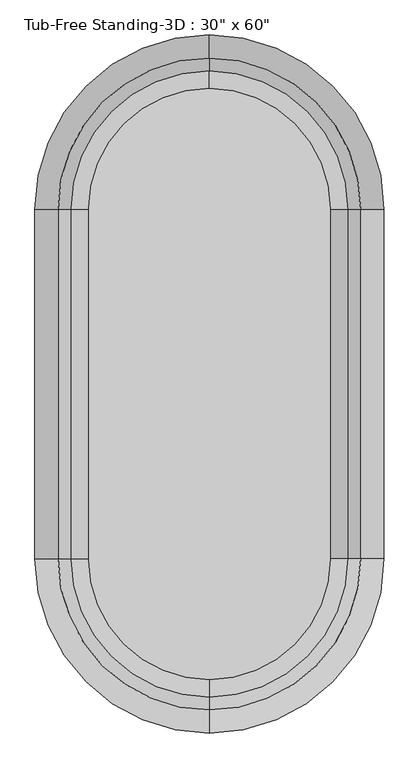
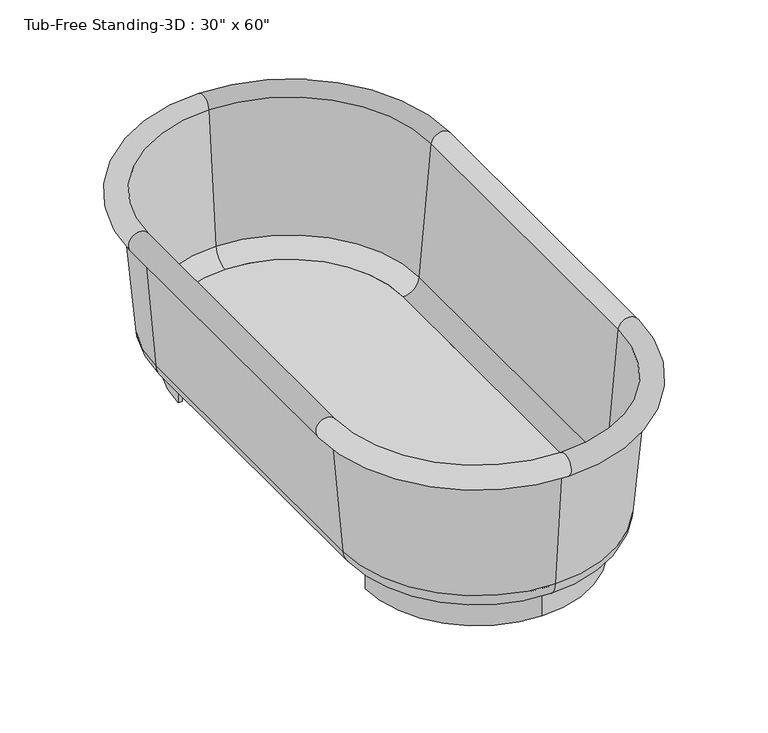
"""IFC4 building model written with IfcOpenShell, lengths in millimetres: flow terminal geometry."""

from ifc_helpers import new_model, si_unit, point, frame, frame_2d, origin, origin_with_axes, place, context, project, spatial, polyline, circle_curve, ellipse_curve, trimmed, segment, composite_curve, outline, extrude, source, transform, mapped, element, save
from ifc_brep_helpers import plane_surface, cylinder_surface, revolved_surface, advanced_brep


def flow_terminal_ce36f001(model_context):
    return source(origin(), model_context, "Body", "SolidModel", [
        advanced_brep(
        [(0.0, 723.9, 406.4), (0.0, 736.6, 406.4), (355.6, 381.0, 406.4), (342.9, 381.0, 406.4), (0.0, 698.1045038, 111.5561295), (317.1045038, 381.0, 111.5561295), (0.0, 645.2824236, 63.1536107), (264.2824236, 381.0, 63.1536107), (0.0, 645.2824236, 78.0774627), (264.2824236, 381.0, 78.0774627), (0.0, 683.2374416, 112.8568289), (302.2374416, 381.0, 112.8568289), (0.0, 711.4561556, 435.3982063), (330.4561556, 381.0, 435.3982063), (-342.9, 381.0, 406.4), (-355.6, 381.0, 406.4), (-317.1045038, 381.0, 111.5561295), (-264.2824236, 381.0, 63.1536107), (-264.2824236, 381.0, 78.0774627), (-302.2374416, 381.0, 112.8568289), (-330.4561556, 381.0, 435.3982063), (-342.9, -381.0, 406.4), (-355.6, -381.0, 406.4), (-317.1045038, -381.0, 111.5561295), (-264.2824236, -381.0, 63.1536107), (-264.2824236, -381.0, 78.0774627), (-302.2374416, -381.0, 112.8568289), (-330.4561556, -381.0, 435.3982063), (0.0, -723.9, 406.4), (0.0, -736.6, 406.4), (0.0, -698.1045038, 111.5561295), (0.0, -645.2824236, 63.1536107), (0.0, -645.2824236, 78.0774627), (0.0, -683.2374416, 112.8568289), (0.0, -711.4561556, 435.3982063), (342.9, -381.0, 406.4), (355.6, -381.0, 406.4), (317.1045038, -381.0, 111.5561295), (264.2824236, -381.0, 63.1536107), (264.2824236, -381.0, 78.0774627), (302.2374416, -381.0, 112.8568289), (330.4561556, -381.0, 435.3982063)],
        [
            (0, 1),
            (1, 2, circle_curve(frame((0.0, 381.0, 406.4), z_axis=(0.0, 0.0, -1.0), x_axis=(1.0, 0.0, 0.0)), 355.6)),
            (2, 3),
            (3, 0, circle_curve(frame((0.0, 381.0, 406.4), z_axis=(0.0, 0.0, 1.0), x_axis=(1.0, 0.0, 0.0)), 342.9)),
            (4, 0),
            (3, 5),
            (5, 4, circle_curve(frame((0.0, 381.0, 111.5561295), z_axis=(0.0, 0.0, 1.0), x_axis=(1.0, 0.0, 0.0)), 317.1045038)),
            (6, 4, circle_curve(frame((0.0, 645.2824236, 116.1774627), z_axis=(1.0, 0.0, 0.0), x_axis=(0.0, 1.0, 0.0)), 53.023852)),
            (5, 7, circle_curve(frame((264.2824236, 381.0, 116.1774627), z_axis=(0.0, 1.0, 0.0), x_axis=(1.0, 0.0, 0.0)), 53.023852)),
            (7, 6, circle_curve(frame((0.0, 381.0, 63.1536107), z_axis=(0.0, 0.0, 1.0), x_axis=(1.0, 0.0, 0.0)), 264.2824236)),
            (8, 6),
            (7, 9),
            (9, 8, circle_curve(frame((0.0, 381.0, 78.0774627), z_axis=(0.0, 0.0, 1.0), x_axis=(1.0, 0.0, 0.0)), 264.2824236)),
            (10, 8, circle_curve(frame((0.0, 645.2824236, 116.1774627), z_axis=(-1.0, 0.0, 0.0), x_axis=(0.0, 1.0, 0.0)), 38.1)),
            (9, 11, circle_curve(frame((264.2824236, 381.0, 116.1774627), z_axis=(0.0, -1.0, 0.0), x_axis=(1.0, 0.0, 0.0)), 38.1)),
            (11, 10, circle_curve(frame((0.0, 381.0, 112.8568289), z_axis=(0.0, 0.0, 1.0), x_axis=(1.0, 0.0, 0.0)), 302.2374416)),
            (12, 10),
            (11, 13),
            (13, 12, circle_curve(frame((0.0, 381.0, 435.3982063), z_axis=(0.0, 0.0, 1.0), x_axis=(1.0, 0.0, 0.0)), 330.4561556)),
            (1, 12, circle_curve(frame((0.0, 736.6, 431.8), z_axis=(1.0, 0.0, 0.0), x_axis=(0.0, 1.0, 0.0)), 25.4)),
            (13, 2, circle_curve(frame((355.6, 381.0, 431.8), z_axis=(0.0, 1.0, 0.0), x_axis=(1.0, 0.0, 0.0)), 25.4)),
            (14, 15),
            (15, 1, circle_curve(frame((0.0, 381.0, 406.4), z_axis=(0.0, 0.0, -1.0), x_axis=(0.0, 1.0, 0.0)), 355.6)),
            (0, 14, circle_curve(frame((0.0, 381.0, 406.4), z_axis=(0.0, 0.0, 1.0), x_axis=(0.0, 1.0, 0.0)), 342.9)),
            (16, 14),
            (4, 16, circle_curve(frame((0.0, 381.0, 111.5561295), z_axis=(0.0, 0.0, 1.0), x_axis=(0.0, 1.0, 0.0)), 317.1045038)),
            (17, 16, circle_curve(frame((-264.2824236, 381.0, 116.1774627), z_axis=(0.0, 1.0, 0.0), x_axis=(-1.0, 0.0, 0.0)), 53.023852)),
            (6, 17, circle_curve(frame((0.0, 381.0, 63.1536107), z_axis=(0.0, 0.0, 1.0), x_axis=(0.0, 1.0, 0.0)), 264.2824236)),
            (18, 17),
            (8, 18, circle_curve(frame((0.0, 381.0, 78.0774627), z_axis=(0.0, 0.0, 1.0), x_axis=(0.0, 1.0, 0.0)), 264.2824236)),
            (19, 18, circle_curve(frame((-264.2824236, 381.0, 116.1774627), z_axis=(0.0, -1.0, 0.0), x_axis=(-1.0, 0.0, 0.0)), 38.1)),
            (10, 19, circle_curve(frame((0.0, 381.0, 112.8568289), z_axis=(0.0, 0.0, 1.0), x_axis=(0.0, 1.0, 0.0)), 302.2374416)),
            (20, 19),
            (12, 20, circle_curve(frame((0.0, 381.0, 435.3982063), z_axis=(0.0, 0.0, 1.0), x_axis=(0.0, 1.0, 0.0)), 330.4561556)),
            (15, 20, circle_curve(frame((-355.6, 381.0, 431.8), z_axis=(0.0, 1.0, 0.0), x_axis=(-1.0, 0.0, 0.0)), 25.4)),
            (14, 21),
            (21, 22),
            (22, 15),
            (16, 23),
            (23, 21),
            (17, 24),
            (24, 23, circle_curve(frame((-264.2824236, -381.0, 116.1774627), z_axis=(0.0, 1.0, 0.0), x_axis=(-1.0, 0.0, 0.0)), 53.023852)),
            (18, 25),
            (25, 24),
            (19, 26),
            (26, 25, circle_curve(frame((-264.2824236, -381.0, 116.1774627), z_axis=(0.0, -1.0, 0.0), x_axis=(-1.0, 0.0, 0.0)), 38.1)),
            (20, 27),
            (27, 26),
            (22, 27, circle_curve(frame((-355.6, -381.0, 431.8), z_axis=(0.0, 1.0, 0.0), x_axis=(-1.0, 0.0, 0.0)), 25.4)),
            (28, 29),
            (29, 22, circle_curve(frame((0.0, -381.0, 406.4), z_axis=(0.0, 0.0, -1.0), x_axis=(-1.0, 0.0, 0.0)), 355.6)),
            (21, 28, circle_curve(frame((0.0, -381.0, 406.4), z_axis=(0.0, 0.0, 1.0), x_axis=(-1.0, 0.0, 0.0)), 342.9)),
            (30, 28),
            (23, 30, circle_curve(frame((0.0, -381.0, 111.5561295), z_axis=(0.0, 0.0, 1.0), x_axis=(-1.0, 0.0, 0.0)), 317.1045038)),
            (31, 30, circle_curve(frame((0.0, -645.2824236, 116.1774627), z_axis=(-1.0, 0.0, 0.0), x_axis=(0.0, -1.0, 0.0)), 53.023852)),
            (24, 31, circle_curve(frame((0.0, -381.0, 63.1536107), z_axis=(0.0, 0.0, 1.0), x_axis=(-1.0, 0.0, 0.0)), 264.2824236)),
            (32, 31),
            (25, 32, circle_curve(frame((0.0, -381.0, 78.0774627), z_axis=(0.0, 0.0, 1.0), x_axis=(-1.0, 0.0, 0.0)), 264.2824236)),
            (33, 32, circle_curve(frame((0.0, -645.2824236, 116.1774627), z_axis=(1.0, 0.0, 0.0), x_axis=(0.0, -1.0, 0.0)), 38.1)),
            (26, 33, circle_curve(frame((0.0, -381.0, 112.8568289), z_axis=(0.0, 0.0, 1.0), x_axis=(-1.0, 0.0, 0.0)), 302.2374416)),
            (34, 33),
            (27, 34, circle_curve(frame((0.0, -381.0, 435.3982063), z_axis=(0.0, 0.0, 1.0), x_axis=(-1.0, 0.0, 0.0)), 330.4561556)),
            (29, 34, circle_curve(frame((0.0, -736.6, 431.8), z_axis=(-1.0, 0.0, 0.0), x_axis=(0.0, -1.0, 0.0)), 25.4)),
            (35, 36),
            (36, 29, circle_curve(frame((0.0, -381.0, 406.4), z_axis=(0.0, 0.0, -1.0), x_axis=(0.0, -1.0, 0.0)), 355.6)),
            (28, 35, circle_curve(frame((0.0, -381.0, 406.4), z_axis=(0.0, 0.0, 1.0), x_axis=(0.0, -1.0, 0.0)), 342.9)),
            (37, 35),
            (30, 37, circle_curve(frame((0.0, -381.0, 111.5561295), z_axis=(0.0, 0.0, 1.0), x_axis=(0.0, -1.0, 0.0)), 317.1045038)),
            (38, 37, circle_curve(frame((264.2824236, -381.0, 116.1774627), z_axis=(0.0, -1.0, 0.0), x_axis=(1.0, 0.0, 0.0)), 53.023852)),
            (31, 38, circle_curve(frame((0.0, -381.0, 63.1536107), z_axis=(0.0, 0.0, 1.0), x_axis=(0.0, -1.0, 0.0)), 264.2824236)),
            (39, 38),
            (32, 39, circle_curve(frame((0.0, -381.0, 78.0774627), z_axis=(0.0, 0.0, 1.0), x_axis=(0.0, -1.0, 0.0)), 264.2824236)),
            (40, 39, circle_curve(frame((264.2824236, -381.0, 116.1774627), z_axis=(0.0, 1.0, 0.0), x_axis=(1.0, 0.0, 0.0)), 38.1)),
            (33, 40, circle_curve(frame((0.0, -381.0, 112.8568289), z_axis=(0.0, 0.0, 1.0), x_axis=(0.0, -1.0, 0.0)), 302.2374416)),
            (41, 40),
            (34, 41, circle_curve(frame((0.0, -381.0, 435.3982063), z_axis=(0.0, 0.0, 1.0), x_axis=(0.0, -1.0, 0.0)), 330.4561556)),
            (36, 41, circle_curve(frame((355.6, -381.0, 431.8), z_axis=(0.0, -1.0, 0.0), x_axis=(1.0, 0.0, 0.0)), 25.4)),
            (35, 3),
            (2, 36),
            (37, 5),
            (38, 7),
            (39, 9),
            (40, 11),
            (41, 13),
        ],
        [
            plane_surface(frame((0.0, 381.0, 406.4), z_axis=(0.0, 0.0, -1.0), x_axis=(1.0, 0.0, 0.0))),
            revolved_surface(polyline([(342.9, 381.0, 406.4), (317.1045038, 381.0, 111.5561295)]), (0.0, 381.0, 431.8), (0.0, 0.0, -1.0)),
            revolved_surface(trimmed(ellipse_curve(frame((264.2824236, 381.0, 116.1774627), z_axis=(0.0, 1.0, 0.0), x_axis=(1.0, 0.0, 0.0)), 53.023852, 53.023852), [point((317.1045038, 381.0, 111.5561295))], [point((264.2824236, 381.0, 63.1536107))], True, "CARTESIAN"), (0.0, 381.0, 431.8), (0.0, 0.0, -1.0)),
            revolved_surface(polyline([(264.2824236, 381.0, 63.1536107), (264.2824236, 381.0, 78.07746270000001)]), (0.0, 381.0, 431.8), (0.0, 0.0, -1.0)),
            revolved_surface(trimmed(ellipse_curve(frame((264.2824236, 381.0, 116.1774627), z_axis=(0.0, -1.0, 0.0), x_axis=(1.0, 0.0, 0.0)), 38.1, 38.1), [point((264.2824236, 381.0, 78.0774627))], [point((302.2374416, 381.0, 112.8568289))], True, "CARTESIAN"), (0.0, 381.0, 431.8), (0.0, 0.0, -1.0)),
            revolved_surface(polyline([(302.2374416, 381.0, 112.8568289), (330.4561556, 381.0, 435.3982063)]), (0.0, 381.0, 431.8), (0.0, 0.0, -1.0)),
            revolved_surface(trimmed(ellipse_curve(frame((355.6, 381.0, 431.8), z_axis=(0.0, 1.0, 0.0), x_axis=(1.0, 0.0, 0.0)), 25.4, 25.4), [point((330.4561556, 381.0, 435.3982063))], [point((355.6, 381.0, 406.4))], True, "CARTESIAN"), (0.0, 381.0, 431.8), (0.0, 0.0, -1.0)),
            plane_surface(frame((0.0, 381.0, 406.4), z_axis=(0.0, 0.0, -1.0), x_axis=(0.0, 1.0, 0.0))),
            revolved_surface(polyline([(0.0, 723.9, 406.4), (0.0, 698.1045038, 111.5561295)]), (0.0, 381.0, 431.8), (0.0, 0.0, -1.0)),
            revolved_surface(trimmed(ellipse_curve(frame((0.0, 645.2824236, 116.1774627), z_axis=(-1.0, 0.0, 0.0), x_axis=(0.0, 1.0, 0.0)), 53.023852, 53.023852), [point((0.0, 698.1045038, 111.5561295))], [point((0.0, 645.2824236, 63.1536107))], True, "CARTESIAN"), (0.0, 381.0, 431.8), (0.0, 0.0, -1.0)),
            revolved_surface(polyline([(0.0, 645.2824236, 63.1536107), (0.0, 645.2824236, 78.07746270000001)]), (0.0, 381.0, 431.8), (0.0, 0.0, -1.0)),
            revolved_surface(trimmed(ellipse_curve(frame((0.0, 645.2824236, 116.1774627), z_axis=(1.0, 0.0, 0.0), x_axis=(0.0, 1.0, 0.0)), 38.1, 38.1), [point((0.0, 645.2824236, 78.0774627))], [point((0.0, 683.2374416, 112.8568289))], True, "CARTESIAN"), (0.0, 381.0, 431.8), (0.0, 0.0, -1.0)),
            revolved_surface(polyline([(0.0, 683.2374416, 112.8568289), (0.0, 711.4561556, 435.3982063)]), (0.0, 381.0, 431.8), (0.0, 0.0, -1.0)),
            revolved_surface(trimmed(ellipse_curve(frame((0.0, 736.6, 431.8), z_axis=(-1.0, 0.0, 0.0), x_axis=(0.0, 1.0, 0.0)), 25.4, 25.4), [point((0.0, 711.4561556, 435.3982063))], [point((0.0, 736.6, 406.4))], True, "CARTESIAN"), (0.0, 381.0, 431.8), (0.0, 0.0, -1.0)),
            plane_surface(frame((-355.6, 381.0, 406.4), z_axis=(0.0, 0.0, -1.0), x_axis=(0.0, -1.0, 0.0))),
            plane_surface(frame((-342.9, 381.0, 406.4), z_axis=(-0.9961946980917455, 0.0, -0.08715574274765871), x_axis=(0.0, -1.0, 0.0))),
            cylinder_surface(frame((-264.2824236, 381.0, 116.1774627), z_axis=(0.0, 1.0, 0.0), x_axis=(-1.0, 0.0, 0.0)), 53.023852),
            plane_surface(frame((-264.2824236, 381.0, 63.1536107), z_axis=(1.0, 0.0, 0.0), x_axis=(0.0, -1.0, 0.0))),
            revolved_surface(polyline([(-302.38242360000004, -381.0, 116.1774627), (-302.38242360000004, 381.0, 116.1774627)]), (-264.2824236, 381.0, 116.1774627), (0.0, -1.0, 0.0)),
            plane_surface(frame((-302.2374416, 381.0, 112.8568289), z_axis=(0.9961946980917458, 0.0, 0.08715574274765651), x_axis=(0.0, -1.0, 0.0))),
            cylinder_surface(frame((-355.6, 381.0, 431.8), z_axis=(0.0, 1.0, 0.0), x_axis=(-1.0, 0.0, 0.0)), 25.4),
            plane_surface(frame((0.0, -381.0, 406.4), z_axis=(0.0, 0.0, -1.0), x_axis=(-1.0, 0.0, 0.0))),
            revolved_surface(polyline([(-342.9, -381.0, 406.4), (-317.1045038, -381.0, 111.5561295)]), (0.0, -381.0, 431.8), (0.0, 0.0, -1.0)),
            revolved_surface(trimmed(ellipse_curve(frame((-264.2824236, -381.0, 116.1774627), z_axis=(0.0, -1.0, 0.0), x_axis=(-1.0, 0.0, 0.0)), 53.023852, 53.023852), [point((-317.1045038, -381.0, 111.5561295))], [point((-264.2824236, -381.0, 63.1536107))], True, "CARTESIAN"), (0.0, -381.0, 431.8), (0.0, 0.0, -1.0)),
            revolved_surface(polyline([(-264.2824236, -381.0, 63.1536107), (-264.2824236, -381.0, 78.07746270000001)]), (0.0, -381.0, 431.8), (0.0, 0.0, -1.0)),
            revolved_surface(trimmed(ellipse_curve(frame((-264.2824236, -381.0, 116.1774627), z_axis=(0.0, 1.0, 0.0), x_axis=(-1.0, 0.0, 0.0)), 38.1, 38.1), [point((-264.2824236, -381.0, 78.0774627))], [point((-302.2374416, -381.0, 112.8568289))], True, "CARTESIAN"), (0.0, -381.0, 431.8), (0.0, 0.0, -1.0)),
            revolved_surface(polyline([(-302.2374416, -381.0, 112.8568289), (-330.4561556, -381.0, 435.3982063)]), (0.0, -381.0, 431.8), (0.0, 0.0, -1.0)),
            revolved_surface(trimmed(ellipse_curve(frame((-355.6, -381.0, 431.8), z_axis=(0.0, -1.0, 0.0), x_axis=(-1.0, 0.0, 0.0)), 25.4, 25.4), [point((-330.4561556, -381.0, 435.3982063))], [point((-355.6, -381.0, 406.4))], True, "CARTESIAN"), (0.0, -381.0, 431.8), (0.0, 0.0, -1.0)),
            plane_surface(frame((0.0, -381.0, 406.4), z_axis=(0.0, 0.0, -1.0), x_axis=(0.0, -1.0, 0.0))),
            revolved_surface(polyline([(0.0, -723.9, 406.4), (0.0, -698.1045038, 111.5561295)]), (0.0, -381.0, 431.8), (0.0, 0.0, -1.0)),
            revolved_surface(trimmed(ellipse_curve(frame((0.0, -645.2824236, 116.1774627), z_axis=(1.0, 0.0, 0.0), x_axis=(0.0, -1.0, 0.0)), 53.023852, 53.023852), [point((0.0, -698.1045038, 111.5561295))], [point((0.0, -645.2824236, 63.1536107))], True, "CARTESIAN"), (0.0, -381.0, 431.8), (0.0, 0.0, -1.0)),
            revolved_surface(polyline([(0.0, -645.2824236, 63.1536107), (0.0, -645.2824236, 78.07746270000001)]), (0.0, -381.0, 431.8), (0.0, 0.0, -1.0)),
            revolved_surface(trimmed(ellipse_curve(frame((0.0, -645.2824236, 116.1774627), z_axis=(-1.0, 0.0, 0.0), x_axis=(0.0, -1.0, 0.0)), 38.1, 38.1), [point((0.0, -645.2824236, 78.0774627))], [point((0.0, -683.2374416, 112.8568289))], True, "CARTESIAN"), (0.0, -381.0, 431.8), (0.0, 0.0, -1.0)),
            revolved_surface(polyline([(0.0, -683.2374416, 112.8568289), (0.0, -711.4561556, 435.3982063)]), (0.0, -381.0, 431.8), (0.0, 0.0, -1.0)),
            revolved_surface(trimmed(ellipse_curve(frame((0.0, -736.6, 431.8), z_axis=(1.0, 0.0, 0.0), x_axis=(0.0, -1.0, 0.0)), 25.4, 25.4), [point((0.0, -711.4561556, 435.3982063))], [point((0.0, -736.6, 406.4))], True, "CARTESIAN"), (0.0, -381.0, 431.8), (0.0, 0.0, -1.0)),
            plane_surface(frame((355.6, -381.0, 406.4), z_axis=(0.0, 0.0, -1.0), x_axis=(0.0, 1.0, 0.0))),
            plane_surface(frame((342.9, -381.0, 406.4), z_axis=(0.9961946980917455, 0.0, -0.08715574274765871), x_axis=(0.0, 1.0, 0.0))),
            cylinder_surface(frame((264.2824236, -381.0, 116.1774627), z_axis=(0.0, -1.0, 0.0), x_axis=(1.0, 0.0, 0.0)), 53.023852),
            plane_surface(frame((264.2824236, -381.0, 63.1536107), z_axis=(-1.0, 0.0, 0.0), x_axis=(0.0, 1.0, 0.0))),
            revolved_surface(polyline([(302.38242360000004, 381.0, 116.1774627), (302.38242360000004, -381.0, 116.1774627)]), (264.2824236, -381.0, 116.1774627), (0.0, 1.0, 0.0)),
            plane_surface(frame((302.2374416, -381.0, 112.8568289), z_axis=(-0.9961946980917458, 0.0, 0.08715574274765651), x_axis=(0.0, 1.0, 0.0))),
            cylinder_surface(frame((355.6, -381.0, 431.8), z_axis=(0.0, -1.0, 0.0), x_axis=(1.0, 0.0, 0.0)), 25.4),
        ],
        [
            (0, [[1, 2, 3, 4]]),
            (1, [[5, -4, 6, 7]]),
            (2, [[8, -7, 9, 10]]),
            (3, [[11, -10, 12, 13]]),
            (4, [[14, -13, 15, 16]]),
            (5, [[17, -16, 18, 19]]),
            (6, [[20, -19, 21, -2]]),
            (7, [[22, 23, -1, 24]]),
            (8, [[25, -24, -5, 26]]),
            (9, [[27, -26, -8, 28]]),
            (10, [[29, -28, -11, 30]]),
            (11, [[31, -30, -14, 32]]),
            (12, [[33, -32, -17, 34]]),
            (13, [[35, -34, -20, -23]]),
            (14, [[36, 37, 38, -22]]),
            (15, [[39, 40, -36, -25]]),
            (16, [[41, 42, -39, -27]]),
            (17, [[43, 44, -41, -29]]),
            (18, [[45, 46, -43, -31]]),
            (19, [[47, 48, -45, -33]]),
            (20, [[-38, 49, -47, -35]]),
            (21, [[50, 51, -37, 52]]),
            (22, [[53, -52, -40, 54]]),
            (23, [[55, -54, -42, 56]]),
            (24, [[57, -56, -44, 58]]),
            (25, [[59, -58, -46, 60]]),
            (26, [[61, -60, -48, 62]]),
            (27, [[63, -62, -49, -51]]),
            (28, [[64, 65, -50, 66]]),
            (29, [[67, -66, -53, 68]]),
            (30, [[69, -68, -55, 70]]),
            (31, [[71, -70, -57, 72]]),
            (32, [[73, -72, -59, 74]]),
            (33, [[75, -74, -61, 76]]),
            (34, [[77, -76, -63, -65]]),
            (35, [[78, -3, 79, -64]]),
            (36, [[80, -6, -78, -67]]),
            (37, [[81, -9, -80, -69]]),
            (38, [[82, -12, -81, -71]]),
            (39, [[83, -15, -82, -73]]),
            (40, [[84, -18, -83, -75]]),
            (41, [[-79, -21, -84, -77]]),
        ],
    ),
        extrude(outline(composite_curve([segment(trimmed(circle_curve(frame_2d((0.0, 381.0)), 264.2824236), [point((-264.2824236, 381.0))], [point((0.0, 645.2824236))], False, "CARTESIAN"), True, "CONTINUOUS"), segment(trimmed(circle_curve(frame_2d((0.0, 381.0)), 264.2824236), [point((0.0, 645.2824236))], [point((264.2824236, 381.0))], False, "CARTESIAN"), True, "CONTINUOUS"), segment(polyline([(264.2824236, 381.0), (264.2824236, -381.0)]), True, "CONTINUOUS"), segment(trimmed(circle_curve(frame_2d((0.0, -381.0)), 264.2824236), [point((264.2824236, -381.0))], [point((0.0, -645.2824236))], False, "CARTESIAN"), True, "CONTINUOUS"), segment(trimmed(circle_curve(frame_2d((0.0, -381.0)), 264.2824236), [point((0.0, -645.2824236))], [point((-264.2824236, -381.0))], False, "CARTESIAN"), True, "CONTINUOUS"), segment(polyline([(-264.2824236, -381.0), (-264.2824236, 381.0)]), True, "CONTINUOUS")], self_intersect=False)), frame((0.0, 0.0, 63.5), z_axis=(0.0, 0.0, 1.0), x_axis=(1.0, 0.0, 0.0)), (0.0, 0.0, 1.0), 15.08125),
        extrude(outline(composite_curve([segment(trimmed(circle_curve(frame_2d((0.0, 381.0)), 264.2824236), [point((0.0, 645.2824236))], [point((264.2824236, 381.0))], False, "CARTESIAN"), True, "CONTINUOUS"), segment(polyline([(264.2824236, 381.0), (254.0, 381.0)]), True, "CONTINUOUS"), segment(trimmed(circle_curve(frame_2d((0.0, 381.0)), 254.0), [point((254.0, 381.0))], [point((0.0, 635.0))], True, "CARTESIAN"), True, "CONTINUOUS"), segment(trimmed(circle_curve(frame_2d((0.0, 381.0)), 254.0), [point((0.0, 635.0))], [point((-254.0, 381.0))], True, "CARTESIAN"), True, "CONTINUOUS"), segment(polyline([(-254.0, 381.0), (-264.2824236, 381.0)]), True, "CONTINUOUS"), segment(trimmed(circle_curve(frame_2d((0.0, 381.0)), 264.2824236), [point((-264.2824236, 381.0))], [point((0.0, 645.2824236))], False, "CARTESIAN"), True, "CONTINUOUS")], self_intersect=False)), origin_with_axes(), (0.0, 0.0, 1.0), 63.5),
        extrude(outline(composite_curve([segment(trimmed(circle_curve(frame_2d((0.0, -381.0)), 254.0), [point((0.0, -635.0))], [point((254.0, -381.0))], True, "CARTESIAN"), True, "CONTINUOUS"), segment(polyline([(254.0, -381.0), (264.2824236, -381.0)]), True, "CONTINUOUS"), segment(trimmed(circle_curve(frame_2d((0.0, -381.0)), 264.2824236), [point((264.2824236, -381.0))], [point((0.0, -645.2824236))], False, "CARTESIAN"), True, "CONTINUOUS"), segment(trimmed(circle_curve(frame_2d((0.0, -381.0)), 264.2824236), [point((0.0, -645.2824236))], [point((-264.2824236, -381.0))], False, "CARTESIAN"), True, "CONTINUOUS"), segment(polyline([(-264.2824236, -381.0), (-254.0, -381.0)]), True, "CONTINUOUS"), segment(trimmed(circle_curve(frame_2d((0.0, -381.0)), 254.0), [point((-254.0, -381.0))], [point((0.0, -635.0))], True, "CARTESIAN"), True, "CONTINUOUS")], self_intersect=False)), origin_with_axes(), (0.0, 0.0, 1.0), 63.5),
    ])


if __name__ == "__main__":
    model = new_model("IFC4")
    model_context = context("Model", 3, world=origin())
    ifc_project = project(units=[si_unit("LENGTHUNIT", "METRE", prefix="MILLI")], contexts=[model_context])
    site = spatial("IfcSite", under=ifc_project)
    building = spatial("IfcBuilding", under=site)
    placement = place(None, origin())
    flow_terminal_shape = flow_terminal_ce36f001(model_context)
    element("IfcFlowTerminal", 1, ObjectType="Tub-Free Standing-3D : 30\" x 60\"", at=placement, inside=building, context=model_context, shape_type="MappedRepresentation", body=[
        mapped(flow_terminal_shape, transform((0.0, 0.0, 0.0), x_axis=(1.0, 0.0, 0.0), y_axis=(0.0, 1.0, 0.0), z_axis=(0.0, 0.0, 1.0))),
    ])
    save(model, "model.ifc")

# Revit data of these elements
# Type "Tub-Free Standing-3D : 30\" x 60\""
#   Assembly Code = "D2010110"
#   Height = 1' - 6"
#   Length = 5' - 0"
#   Width = 2' - 6"
#   Tub Material = Porcelain, Ivory
#   Default Elevation = 0
# Element 1 (IfcFlowTerminal, "Tub-Free Standing-3D : 30\" x 60\"")
#   Materials on its faces: "Porcelain, Ivory"
# Materials
#   "Porcelain, Ivory": class "Ceramic", colour RGB 247 247 239, transparency 0, Description = "Porcelain, ivory", Cost = 0
